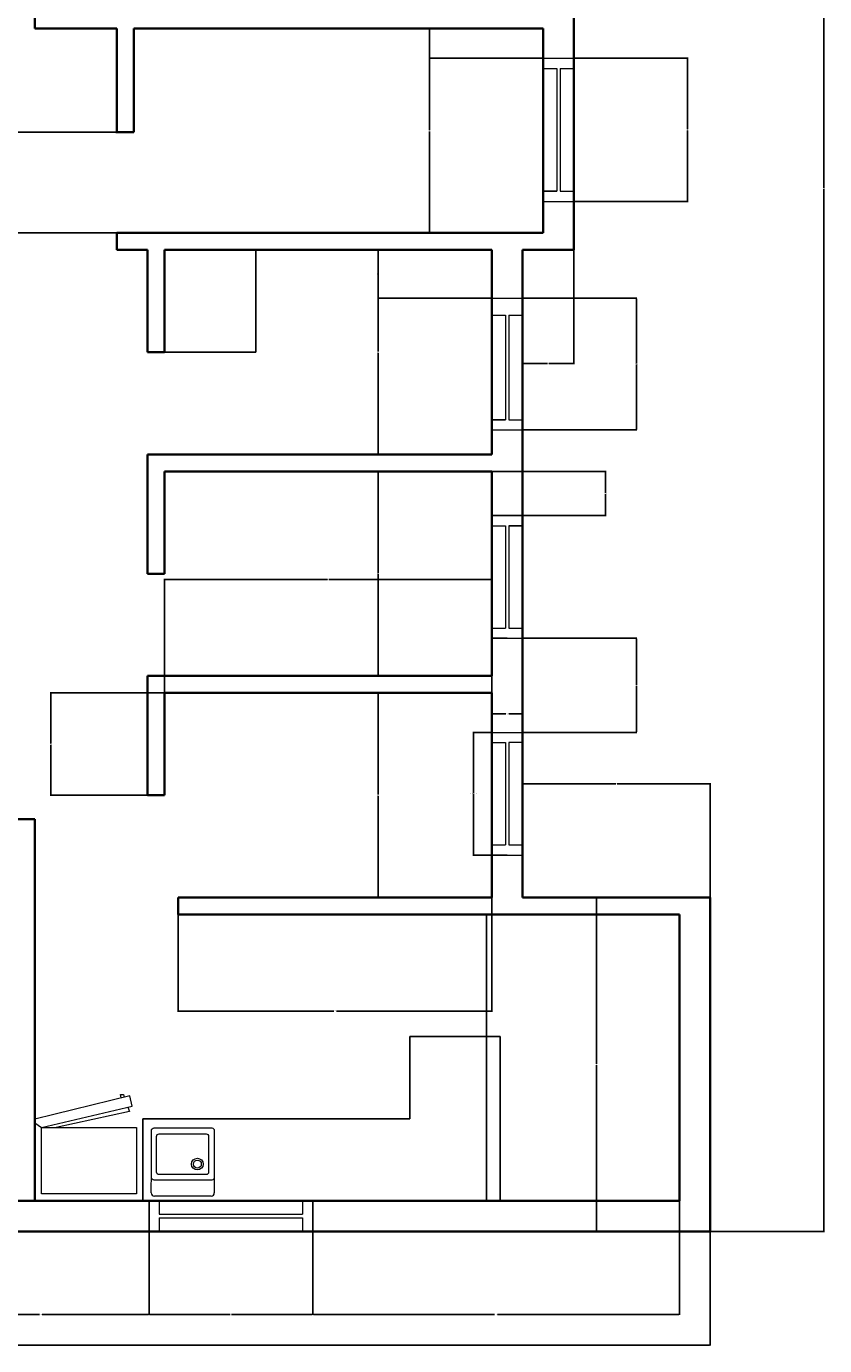
# Model space of a CAD drawing. Units: inches. Extents: x 1201 to 1750, y 1179 to 1858.
# Tile 2 of 3: x 1515 to 1750, y 1179 to 1566. Entities that reach past the tile are written whole.
import ezdxf

# ---------------------------------------------------------------- set-up
doc = ezdxf.new("R2010")
doc.units = ezdxf.units.IN
for name, color, linetype, lineweight in [('A-ANNO-DIMS', 2, 'Continuous', 18), ('A-EQPM', 8, 'Continuous', 18), ('A-FLOR-CASE', 9, 'Continuous', 25), ('A-FLOR-FIXT', 9, 'Continuous', 18), ('A-GLAZ', 4, 'Continuous', 18), ('A-WALL', 7, 'Continuous', 35)]:
    doc.layers.add(name, color=color, linetype=linetype, lineweight=lineweight)
doc.styles.get("Standard").update_dxf_attribs({"font": 'times.ttf'})
doc.dimstyles.get("Standard").update_dxf_attribs({"dimtxt": 0.18, "dimasz": 0.18, "dimexe": 0.18, "dimexo": 0.0625, "dimgap": 0.09, "dimtad": 0, "dimtih": 1, "dimtoh": 1, "dimdec": 4, "dimzin": 0, "dimdsep": 46, "dimtxsty": 'Standard', "dimcen": 0.09, "dimadec": 0, "dimazin": 0, "dimtfac": 1, "dimtdec": 4, "dimtofl": 0, "dimtmove": 0, "dimatfit": 3, "dimfxl": 1, "dimtolj": 1, "dimtzin": 0, "dimarcsym": 0})

# ---------------------------------------------------------------- blocks, each defined once
blk = doc.blocks.new('WIN-36IN')
for p, q in [((0, 36), (9, 36)), ((0, 33), (4, 33)), ((4, 33), (4, 3)), ((9, 33), (5, 33)), ((5, 33), (5, 3)), ((0, 3), (4, 3)), ((5, 3), (9, 3)), ((0, 0), (9, 0)), ((4.5, 0), (0, 0))]:
    blk.add_line(p, q)
blk = doc.blocks.new('*D5')
at = {"layer": 'A-ANNO-DIMS', "color": 0, "lineweight": -2, "transparency": 16777216}
for p, q in [((1651.92, 1358.68), (1646.41, 1358.68)), ((1646.59, 1358.5), (1646.59, 1340.86)), ((1646.59, 1322.86), (1646.59, 1340.5)), ((1651.92, 1322.68), (1646.41, 1322.68))]:
    blk.add_line(p, q, dxfattribs=at)
at = {"layer": 'A-ANNO-DIMS', "color": 0, "transparency": 16777216}
for points in [[(1646.56, 1358.5), (1646.62, 1358.5), (1646.59, 1358.68)], [(1646.56, 1322.86), (1646.62, 1322.86), (1646.59, 1322.68)]]:
    blk.add_solid(points, dxfattribs=at)
at = {"layer": 'Defpoints', "color": 0, "transparency": 16777216}
for p in [(1646.59, 1358.68), (1651.99, 1358.68), (1651.99, 1322.68)]:
    blk.add_point(p, dxfattribs=at)
at = {"layer": 'A-ANNO-DIMS', "color": 0, "transparency": 16777216, "insert": (1646.59, 1340.68), "char_height": 0.18, "attachment_point": 5}
blk.add_mtext('\\A1;WINDOW 36 TYP.', dxfattribs=at)
blk = doc.blocks.new('*D6')
at = {"layer": 'A-ANNO-DIMS', "color": 0, "lineweight": -2, "transparency": 16777216}
for p, q in [((1651.99, 1358.74), (1651.99, 1364.26)), ((1652.17, 1364.08), (1656.03, 1364.08)), ((1660.81, 1364.08), (1656.95, 1364.08)), ((1660.99, 1358.74), (1660.99, 1364.26))]:
    blk.add_line(p, q, dxfattribs=at)
at = {"layer": 'A-ANNO-DIMS', "color": 0, "transparency": 16777216}
for points in [[(1652.17, 1364.11), (1652.17, 1364.05), (1651.99, 1364.08)], [(1660.81, 1364.11), (1660.81, 1364.05), (1660.99, 1364.08)]]:
    blk.add_solid(points, dxfattribs=at)
at = {"layer": 'Defpoints', "color": 0, "transparency": 16777216}
for p in [(1660.99, 1364.08), (1651.99, 1358.68), (1660.99, 1358.68)]:
    blk.add_point(p, dxfattribs=at)
at = {"layer": 'A-ANNO-DIMS', "color": 0, "transparency": 16777216, "insert": (1656.49, 1364.08), "char_height": 0.18, "attachment_point": 5}
blk.add_mtext('\\A1;9 TYP.', dxfattribs=at)
blk = doc.blocks.new('*D7')
at = {"layer": 'A-ANNO-DIMS', "color": 0, "lineweight": -2, "transparency": 16777216}
for p, q in [((1234.99, 1212.18), (1234.99, 1178.71)), ((1715.99, 1212.18), (1715.99, 1178.71)), ((1235.17, 1178.89), (1475.22, 1178.89)), ((1715.81, 1178.89), (1475.76, 1178.89))]:
    blk.add_line(p, q, dxfattribs=at)
at = {"layer": 'A-ANNO-DIMS', "color": 0, "transparency": 16777216}
for points in [[(1235.17, 1178.92), (1235.17, 1178.86), (1234.99, 1178.89)], [(1715.81, 1178.92), (1715.81, 1178.86), (1715.99, 1178.89)]]:
    blk.add_solid(points, dxfattribs=at)
at = {"layer": 'Defpoints', "color": 0, "transparency": 16777216}
for p in [(1234.99, 1212.24), (1715.99, 1212.24), (1234.99, 1178.89)]:
    blk.add_point(p, dxfattribs=at)
at = {"layer": 'A-ANNO-DIMS', "color": 0, "transparency": 16777216, "insert": (1475.49, 1178.89), "char_height": 0.18, "attachment_point": 5}
blk.add_mtext('\\A1;481', dxfattribs=at)
blk = doc.blocks.new('*D8')
at = {"layer": 'A-ANNO-DIMS', "color": 0, "lineweight": -2, "transparency": 16777216}
for p, q in [((1676.05, 1824.24), (1749.52, 1824.24)), ((1749.34, 1824.06), (1749.34, 1518.42)), ((1749.34, 1212.42), (1749.34, 1518.06)), ((1716.05, 1212.24), (1749.52, 1212.24))]:
    blk.add_line(p, q, dxfattribs=at)
at = {"layer": 'A-ANNO-DIMS', "color": 0, "transparency": 16777216}
for points in [[(1749.31, 1824.06), (1749.37, 1824.06), (1749.34, 1824.24)], [(1749.31, 1212.42), (1749.37, 1212.42), (1749.34, 1212.24)]]:
    blk.add_solid(points, dxfattribs=at)
at = {"layer": 'Defpoints', "color": 0, "transparency": 16777216}
for p in [(1675.99, 1824.24), (1749.34, 1824.24), (1715.99, 1212.24)]:
    blk.add_point(p, dxfattribs=at)
at = {"layer": 'A-ANNO-DIMS', "color": 0, "transparency": 16777216, "insert": (1749.34, 1518.24), "char_height": 0.18, "attachment_point": 5}
blk.add_mtext('\\A1;612', dxfattribs=at)
blk = doc.blocks.new('*D14')
at = {"layer": 'A-ANNO-DIMS', "color": 0, "lineweight": -2, "transparency": 16777216}
for p, q in [((1715.92, 1310.24), (1682.46, 1310.24)), ((1682.64, 1310.06), (1682.64, 1261.42)), ((1682.64, 1212.42), (1682.64, 1261.06)), ((1715.92, 1212.24), (1682.46, 1212.24))]:
    blk.add_line(p, q, dxfattribs=at)
at = {"layer": 'A-ANNO-DIMS', "color": 0, "transparency": 16777216}
for points in [[(1682.61, 1310.06), (1682.67, 1310.06), (1682.64, 1310.24)], [(1682.61, 1212.42), (1682.67, 1212.42), (1682.64, 1212.24)]]:
    blk.add_solid(points, dxfattribs=at)
at = {"layer": 'Defpoints', "color": 0, "transparency": 16777216}
for p in [(1682.64, 1310.24), (1715.99, 1310.24), (1715.99, 1212.24)]:
    blk.add_point(p, dxfattribs=at)
at = {"layer": 'A-ANNO-DIMS', "color": 0, "transparency": 16777216, "insert": (1682.64, 1261.24), "char_height": 0.18, "attachment_point": 5}
blk.add_mtext('\\A1;98', dxfattribs=at)
blk = doc.blocks.new('*D15')
at = {"layer": 'A-ANNO-DIMS', "color": 0, "lineweight": -2, "transparency": 16777216}
for p, q in [((1660.99, 1310.3), (1660.99, 1343.77)), ((1661.17, 1343.59), (1688.28, 1343.59)), ((1715.81, 1343.59), (1688.69, 1343.59)), ((1715.99, 1310.3), (1715.99, 1343.77))]:
    blk.add_line(p, q, dxfattribs=at)
at = {"layer": 'A-ANNO-DIMS', "color": 0, "transparency": 16777216}
for points in [[(1661.17, 1343.62), (1661.17, 1343.56), (1660.99, 1343.59)], [(1715.81, 1343.62), (1715.81, 1343.56), (1715.99, 1343.59)]]:
    blk.add_solid(points, dxfattribs=at)
at = {"layer": 'Defpoints', "color": 0, "transparency": 16777216}
for p in [(1715.99, 1343.59), (1660.99, 1310.24), (1715.99, 1310.24)]:
    blk.add_point(p, dxfattribs=at)
at = {"layer": 'A-ANNO-DIMS', "color": 0, "transparency": 16777216, "insert": (1688.49, 1343.59), "char_height": 0.18, "attachment_point": 5}
blk.add_mtext('\\A1;55', dxfattribs=at)
blk = doc.blocks.new('*D16')
at = {"layer": 'A-ANNO-DIMS', "color": 0, "lineweight": -2, "transparency": 16777216}
for p, q in [((1660.99, 1500.18), (1660.99, 1466.71)), ((1675.99, 1500.18), (1675.99, 1466.71)), ((1661.17, 1466.89), (1668.29, 1466.89)), ((1675.81, 1466.89), (1668.69, 1466.89))]:
    blk.add_line(p, q, dxfattribs=at)
at = {"layer": 'A-ANNO-DIMS', "color": 0, "transparency": 16777216}
for points in [[(1661.17, 1466.92), (1661.17, 1466.86), (1660.99, 1466.89)], [(1675.81, 1466.92), (1675.81, 1466.86), (1675.99, 1466.89)]]:
    blk.add_solid(points, dxfattribs=at)
at = {"layer": 'Defpoints', "color": 0, "transparency": 16777216}
for p in [(1660.99, 1500.24), (1675.99, 1500.24), (1660.99, 1466.89)]:
    blk.add_point(p, dxfattribs=at)
at = {"layer": 'A-ANNO-DIMS', "color": 0, "transparency": 16777216, "insert": (1668.49, 1466.89), "char_height": 0.18, "attachment_point": 5}
blk.add_mtext('\\A1;15', dxfattribs=at)
blk = doc.blocks.new('*D17')
at = {"layer": 'A-ANNO-DIMS', "color": 0, "lineweight": -2, "transparency": 16777216}
for p, q in [((1666.92, 1565.24), (1633.46, 1565.24)), ((1633.64, 1565.06), (1633.64, 1535.42)), ((1633.64, 1505.42), (1633.64, 1535.06)), ((1666.92, 1505.24), (1633.46, 1505.24))]:
    blk.add_line(p, q, dxfattribs=at)
at = {"layer": 'A-ANNO-DIMS', "color": 0, "transparency": 16777216}
for points in [[(1633.61, 1565.06), (1633.67, 1565.06), (1633.64, 1565.24)], [(1633.61, 1505.42), (1633.67, 1505.42), (1633.64, 1505.24)]]:
    blk.add_solid(points, dxfattribs=at)
at = {"layer": 'Defpoints', "color": 0, "transparency": 16777216}
for p in [(1633.64, 1565.24), (1666.99, 1565.24), (1666.99, 1505.24)]:
    blk.add_point(p, dxfattribs=at)
at = {"layer": 'A-ANNO-DIMS', "color": 0, "transparency": 16777216, "insert": (1633.64, 1535.24), "char_height": 0.18, "attachment_point": 5}
blk.add_mtext('\\A1;60', dxfattribs=at)
blk = doc.blocks.new('*D20')
at = {"layer": 'A-ANNO-DIMS', "color": 0, "lineweight": -2, "transparency": 16777216}
for p, q in [((1555.99, 1370.3), (1555.99, 1403.77)), ((1556.17, 1403.59), (1603.77, 1403.59)), ((1651.81, 1403.59), (1604.2, 1403.59)), ((1651.99, 1370.3), (1651.99, 1403.77))]:
    blk.add_line(p, q, dxfattribs=at)
at = {"layer": 'A-ANNO-DIMS', "color": 0, "transparency": 16777216}
for points in [[(1556.17, 1403.62), (1556.17, 1403.56), (1555.99, 1403.59)], [(1651.81, 1403.62), (1651.81, 1403.56), (1651.99, 1403.59)]]:
    blk.add_solid(points, dxfattribs=at)
at = {"layer": 'Defpoints', "color": 0, "transparency": 16777216}
for p in [(1651.99, 1403.59), (1555.99, 1370.24), (1651.99, 1370.24)]:
    blk.add_point(p, dxfattribs=at)
at = {"layer": 'A-ANNO-DIMS', "color": 0, "transparency": 16777216, "insert": (1603.99, 1403.59), "char_height": 0.18, "attachment_point": 5}
blk.add_mtext('\\A1;96', dxfattribs=at)
blk = doc.blocks.new('*D21')
at = {"layer": 'A-ANNO-DIMS', "color": 0, "lineweight": -2, "transparency": 16777216}
for p, q in [((1651.92, 1370.24), (1618.46, 1370.24)), ((1618.64, 1370.06), (1618.64, 1340.42)), ((1618.64, 1310.42), (1618.64, 1340.06)), ((1651.92, 1310.24), (1618.46, 1310.24))]:
    blk.add_line(p, q, dxfattribs=at)
at = {"layer": 'A-ANNO-DIMS', "color": 0, "transparency": 16777216}
for points in [[(1618.61, 1370.06), (1618.67, 1370.06), (1618.64, 1370.24)], [(1618.61, 1310.42), (1618.67, 1310.42), (1618.64, 1310.24)]]:
    blk.add_solid(points, dxfattribs=at)
at = {"layer": 'Defpoints', "color": 0, "transparency": 16777216}
for p in [(1618.64, 1370.24), (1651.99, 1370.24), (1651.99, 1310.24)]:
    blk.add_point(p, dxfattribs=at)
at = {"layer": 'A-ANNO-DIMS', "color": 0, "transparency": 16777216, "insert": (1618.64, 1340.24), "char_height": 0.18, "attachment_point": 5}
blk.add_mtext('\\A1;60', dxfattribs=at)
blk = doc.blocks.new('*D22')
at = {"layer": 'A-ANNO-DIMS', "color": 0, "lineweight": -2, "transparency": 16777216}
for p, q in [((1651.92, 1435.24), (1618.46, 1435.24)), ((1618.64, 1435.06), (1618.64, 1405.42)), ((1618.64, 1375.42), (1618.64, 1405.06)), ((1651.92, 1375.24), (1618.46, 1375.24))]:
    blk.add_line(p, q, dxfattribs=at)
at = {"layer": 'A-ANNO-DIMS', "color": 0, "transparency": 16777216}
for points in [[(1618.61, 1435.06), (1618.67, 1435.06), (1618.64, 1435.24)], [(1618.61, 1375.42), (1618.67, 1375.42), (1618.64, 1375.24)]]:
    blk.add_solid(points, dxfattribs=at)
at = {"layer": 'Defpoints', "color": 0, "transparency": 16777216}
for p in [(1618.64, 1435.24), (1651.99, 1435.24), (1651.99, 1375.24)]:
    blk.add_point(p, dxfattribs=at)
at = {"layer": 'A-ANNO-DIMS', "color": 0, "transparency": 16777216, "insert": (1618.64, 1405.24), "char_height": 0.18, "attachment_point": 5}
blk.add_mtext('\\A1;60', dxfattribs=at)
blk = doc.blocks.new('*D23')
at = {"layer": 'A-ANNO-DIMS', "color": 0, "lineweight": -2, "transparency": 16777216}
for p, q in [((1651.92, 1500.24), (1618.46, 1500.24)), ((1618.64, 1500.06), (1618.64, 1470.42)), ((1618.64, 1440.42), (1618.64, 1470.06)), ((1651.92, 1440.24), (1618.46, 1440.24))]:
    blk.add_line(p, q, dxfattribs=at)
at = {"layer": 'A-ANNO-DIMS', "color": 0, "transparency": 16777216}
for points in [[(1618.61, 1500.06), (1618.67, 1500.06), (1618.64, 1500.24)], [(1618.61, 1440.42), (1618.67, 1440.42), (1618.64, 1440.24)]]:
    blk.add_solid(points, dxfattribs=at)
at = {"layer": 'Defpoints', "color": 0, "transparency": 16777216}
for p in [(1618.64, 1500.24), (1651.99, 1500.24), (1651.99, 1440.24)]:
    blk.add_point(p, dxfattribs=at)
at = {"layer": 'A-ANNO-DIMS', "color": 0, "transparency": 16777216, "insert": (1618.64, 1470.24), "char_height": 0.18, "attachment_point": 5}
blk.add_mtext('\\A1;60', dxfattribs=at)
blk = doc.blocks.new('*D33')
at = {"layer": 'A-ANNO-DIMS', "color": 0, "lineweight": -2, "transparency": 16777216}
for p, q in [((1476.42, 1565.3), (1476.42, 1598.77)), ((1476.6, 1598.59), (1496.82, 1598.59)), ((1517.81, 1598.59), (1497.58, 1598.59)), ((1517.99, 1565.3), (1517.99, 1598.77))]:
    blk.add_line(p, q, dxfattribs=at)
at = {"layer": 'A-ANNO-DIMS', "color": 0, "transparency": 16777216}
for points in [[(1476.6, 1598.62), (1476.6, 1598.56), (1476.42, 1598.59)], [(1517.81, 1598.62), (1517.81, 1598.56), (1517.99, 1598.59)]]:
    blk.add_solid(points, dxfattribs=at)
at = {"layer": 'Defpoints', "color": 0, "transparency": 16777216}
for p in [(1517.99, 1598.59), (1476.42, 1565.24), (1517.99, 1565.24)]:
    blk.add_point(p, dxfattribs=at)
at = {"layer": 'A-ANNO-DIMS', "color": 0, "transparency": 16777216, "insert": (1497.2, 1598.59), "char_height": 0.18, "attachment_point": 5}
blk.add_mtext('\\A1;41.57', dxfattribs=at)
blk = doc.blocks.new('*D42')
at = {"layer": 'A-ANNO-DIMS', "color": 0, "lineweight": -2, "transparency": 16777216}
for p, q in [((1487.97, 1221.18), (1487.97, 1187.71)), ((1551.45, 1221.18), (1551.45, 1187.71)), ((1488.15, 1187.89), (1519.33, 1187.89)), ((1551.27, 1187.89), (1520.09, 1187.89))]:
    blk.add_line(p, q, dxfattribs=at)
at = {"layer": 'A-ANNO-DIMS', "color": 0, "transparency": 16777216}
for points in [[(1488.15, 1187.92), (1488.15, 1187.86), (1487.97, 1187.89)], [(1551.27, 1187.92), (1551.27, 1187.86), (1551.45, 1187.89)]]:
    blk.add_solid(points, dxfattribs=at)
at = {"layer": 'Defpoints', "color": 0, "transparency": 16777216}
for p in [(1487.97, 1221.24), (1551.45, 1221.24), (1487.97, 1187.89)]:
    blk.add_point(p, dxfattribs=at)
at = {"layer": 'A-ANNO-DIMS', "color": 0, "transparency": 16777216, "insert": (1519.71, 1187.89), "char_height": 0.18, "attachment_point": 5}
blk.add_mtext('\\A1;63.48', dxfattribs=at)
blk = doc.blocks.new('*D43')
at = {"layer": 'A-ANNO-DIMS', "color": 0, "lineweight": -2, "transparency": 16777216}
for p, q in [((1551.45, 1221.18), (1551.45, 1187.71)), ((1599.45, 1221.18), (1599.45, 1187.71)), ((1551.63, 1187.89), (1575.23, 1187.89)), ((1599.27, 1187.89), (1575.66, 1187.89))]:
    blk.add_line(p, q, dxfattribs=at)
at = {"layer": 'A-ANNO-DIMS', "color": 0, "transparency": 16777216}
for points in [[(1551.63, 1187.92), (1551.63, 1187.86), (1551.45, 1187.89)], [(1599.27, 1187.92), (1599.27, 1187.86), (1599.45, 1187.89)]]:
    blk.add_solid(points, dxfattribs=at)
at = {"layer": 'Defpoints', "color": 0, "transparency": 16777216}
for p in [(1551.45, 1221.24), (1599.45, 1221.24), (1551.45, 1187.89)]:
    blk.add_point(p, dxfattribs=at)
at = {"layer": 'A-ANNO-DIMS', "color": 0, "transparency": 16777216, "insert": (1575.45, 1187.89), "char_height": 0.18, "attachment_point": 5}
blk.add_mtext('\\A1;48', dxfattribs=at)
blk = doc.blocks.new('*D44')
at = {"layer": 'A-ANNO-DIMS', "color": 0, "lineweight": -2, "transparency": 16777216}
for p, q in [((1599.45, 1221.18), (1599.45, 1187.71)), ((1706.99, 1221.18), (1706.99, 1187.71)), ((1599.63, 1187.89), (1652.78, 1187.89)), ((1706.81, 1187.89), (1653.65, 1187.89))]:
    blk.add_line(p, q, dxfattribs=at)
at = {"layer": 'A-ANNO-DIMS', "color": 0, "transparency": 16777216}
for points in [[(1599.63, 1187.92), (1599.63, 1187.86), (1599.45, 1187.89)], [(1706.81, 1187.92), (1706.81, 1187.86), (1706.99, 1187.89)]]:
    blk.add_solid(points, dxfattribs=at)
at = {"layer": 'Defpoints', "color": 0, "transparency": 16777216}
for p in [(1599.45, 1221.24), (1706.99, 1221.24), (1599.45, 1187.89)]:
    blk.add_point(p, dxfattribs=at)
at = {"layer": 'A-ANNO-DIMS', "color": 0, "transparency": 16777216, "insert": (1653.22, 1187.89), "char_height": 0.18, "attachment_point": 5}
blk.add_mtext('\\A1;107.54', dxfattribs=at)
blk = doc.blocks.new('*D50')
at = {"layer": 'A-ANNO-DIMS', "color": 0, "lineweight": -2, "transparency": 16777216}
for p, q in [((1541.92, 1534.83), (1508.46, 1534.83)), ((1508.64, 1534.65), (1508.64, 1520.22)), ((1508.64, 1505.42), (1508.64, 1519.85)), ((1541.92, 1505.24), (1508.46, 1505.24))]:
    blk.add_line(p, q, dxfattribs=at)
at = {"layer": 'A-ANNO-DIMS', "color": 0, "transparency": 16777216}
for points in [[(1508.61, 1534.65), (1508.67, 1534.65), (1508.64, 1534.83)], [(1508.61, 1505.42), (1508.67, 1505.42), (1508.64, 1505.24)]]:
    blk.add_solid(points, dxfattribs=at)
at = {"layer": 'Defpoints', "color": 0, "transparency": 16777216}
for p in [(1508.64, 1534.83), (1541.99, 1534.83), (1541.99, 1505.24)]:
    blk.add_point(p, dxfattribs=at)
at = {"layer": 'A-ANNO-DIMS', "color": 0, "transparency": 16777216, "insert": (1508.64, 1520.03), "char_height": 0.18, "attachment_point": 5}
blk.add_mtext('\\A1;29.585', dxfattribs=at)
blk = doc.blocks.new('*D51')
at = {"layer": 'A-ANNO-DIMS', "color": 0, "lineweight": -2, "transparency": 16777216}
for p, q in [((1555.92, 1370.24), (1522.46, 1370.24)), ((1522.64, 1370.06), (1522.64, 1355.42)), ((1522.64, 1340.42), (1522.64, 1355.06)), ((1555.92, 1340.24), (1522.46, 1340.24))]:
    blk.add_line(p, q, dxfattribs=at)
at = {"layer": 'A-ANNO-DIMS', "color": 0, "transparency": 16777216}
for points in [[(1522.61, 1370.06), (1522.67, 1370.06), (1522.64, 1370.24)], [(1522.61, 1340.42), (1522.67, 1340.42), (1522.64, 1340.24)]]:
    blk.add_solid(points, dxfattribs=at)
at = {"layer": 'Defpoints', "color": 0, "transparency": 16777216}
for p in [(1522.64, 1370.24), (1555.99, 1370.24), (1555.99, 1340.24)]:
    blk.add_point(p, dxfattribs=at)
at = {"layer": 'A-ANNO-DIMS', "color": 0, "transparency": 16777216, "insert": (1522.64, 1355.24), "char_height": 0.18, "attachment_point": 5}
blk.add_mtext('\\A1;30', dxfattribs=at)
blk = doc.blocks.new('*D52')
at = {"layer": 'A-ANNO-DIMS', "color": 0, "lineweight": -2, "transparency": 16777216}
for p, q in [((1661.05, 1386.31), (1694.52, 1386.31)), ((1694.34, 1386.13), (1694.34, 1372.67)), ((1694.34, 1358.86), (1694.34, 1372.31)), ((1661.05, 1358.68), (1694.52, 1358.68))]:
    blk.add_line(p, q, dxfattribs=at)
at = {"layer": 'A-ANNO-DIMS', "color": 0, "transparency": 16777216}
for points in [[(1694.31, 1386.13), (1694.37, 1386.13), (1694.34, 1386.31)], [(1694.31, 1358.86), (1694.37, 1358.86), (1694.34, 1358.68)]]:
    blk.add_solid(points, dxfattribs=at)
at = {"layer": 'Defpoints', "color": 0, "transparency": 16777216}
for p in [(1660.99, 1386.31), (1660.99, 1358.68), (1694.34, 1358.68)]:
    blk.add_point(p, dxfattribs=at)
at = {"layer": 'A-ANNO-DIMS', "color": 0, "transparency": 16777216, "insert": (1694.34, 1372.49), "char_height": 0.18, "attachment_point": 5}
blk.add_mtext('\\A1;27.63', dxfattribs=at)
blk = doc.blocks.new('*D53')
at = {"layer": 'A-ANNO-DIMS', "color": 0, "lineweight": -2, "transparency": 16777216}
for p, q in [((1652.05, 1435.24), (1685.52, 1435.24)), ((1685.34, 1435.06), (1685.34, 1428.96)), ((1685.34, 1422.49), (1685.34, 1428.59)), ((1652.05, 1422.31), (1685.52, 1422.31))]:
    blk.add_line(p, q, dxfattribs=at)
at = {"layer": 'A-ANNO-DIMS', "color": 0, "transparency": 16777216}
for points in [[(1685.31, 1435.06), (1685.37, 1435.06), (1685.34, 1435.24)], [(1685.31, 1422.49), (1685.37, 1422.49), (1685.34, 1422.31)]]:
    blk.add_solid(points, dxfattribs=at)
at = {"layer": 'Defpoints', "color": 0, "transparency": 16777216}
for p in [(1651.99, 1435.24), (1651.99, 1422.31), (1685.34, 1422.31)]:
    blk.add_point(p, dxfattribs=at)
at = {"layer": 'A-ANNO-DIMS', "color": 0, "transparency": 16777216, "insert": (1685.34, 1428.77), "char_height": 0.18, "attachment_point": 5}
blk.add_mtext('\\A1;12.936', dxfattribs=at)
blk = doc.blocks.new('*D54')
at = {"layer": 'A-ANNO-DIMS', "color": 0, "lineweight": -2, "transparency": 16777216}
for p, q in [((1661.05, 1486.12), (1694.52, 1486.12)), ((1694.34, 1485.94), (1694.34, 1466.95)), ((1694.34, 1447.6), (1694.34, 1466.59)), ((1661.05, 1447.42), (1694.52, 1447.42))]:
    blk.add_line(p, q, dxfattribs=at)
at = {"layer": 'A-ANNO-DIMS', "color": 0, "transparency": 16777216}
for points in [[(1694.31, 1485.94), (1694.37, 1485.94), (1694.34, 1486.12)], [(1694.31, 1447.6), (1694.37, 1447.6), (1694.34, 1447.42)]]:
    blk.add_solid(points, dxfattribs=at)
at = {"layer": 'Defpoints', "color": 0, "transparency": 16777216}
for p in [(1660.99, 1486.12), (1660.99, 1447.42), (1694.34, 1447.42)]:
    blk.add_point(p, dxfattribs=at)
at = {"layer": 'A-ANNO-DIMS', "color": 0, "transparency": 16777216, "insert": (1694.34, 1466.77), "char_height": 0.18, "attachment_point": 5}
blk.add_mtext('\\A1;38.695', dxfattribs=at)
blk = doc.blocks.new('*D55')
at = {"layer": 'A-ANNO-DIMS', "color": 0, "lineweight": -2, "transparency": 16777216}
for p, q in [((1651.92, 1500.24), (1618.46, 1500.24)), ((1618.64, 1500.06), (1618.64, 1493.36)), ((1618.64, 1486.3), (1618.64, 1493)), ((1651.92, 1486.12), (1618.46, 1486.12))]:
    blk.add_line(p, q, dxfattribs=at)
at = {"layer": 'A-ANNO-DIMS', "color": 0, "transparency": 16777216}
for points in [[(1618.61, 1500.06), (1618.67, 1500.06), (1618.64, 1500.24)], [(1618.61, 1486.3), (1618.67, 1486.3), (1618.64, 1486.12)]]:
    blk.add_solid(points, dxfattribs=at)
at = {"layer": 'Defpoints', "color": 0, "transparency": 16777216}
for p in [(1618.64, 1500.24), (1651.99, 1500.24), (1651.99, 1486.12)]:
    blk.add_point(p, dxfattribs=at)
at = {"layer": 'A-ANNO-DIMS', "color": 0, "transparency": 16777216, "insert": (1618.64, 1493.18), "char_height": 0.18, "attachment_point": 5}
blk.add_mtext('\\A1;14.122', dxfattribs=at)
blk = doc.blocks.new('*D56')
at = {"layer": 'A-ANNO-DIMS', "color": 0, "lineweight": -2, "transparency": 16777216}
for p, q in [((1666.92, 1565.24), (1633.46, 1565.24)), ((1633.64, 1565.06), (1633.64, 1561.05)), ((1633.64, 1556.67), (1633.64, 1560.68)), ((1666.92, 1556.49), (1633.46, 1556.49))]:
    blk.add_line(p, q, dxfattribs=at)
at = {"layer": 'A-ANNO-DIMS', "color": 0, "transparency": 16777216}
for points in [[(1633.61, 1565.06), (1633.67, 1565.06), (1633.64, 1565.24)], [(1633.61, 1556.67), (1633.67, 1556.67), (1633.64, 1556.49)]]:
    blk.add_solid(points, dxfattribs=at)
at = {"layer": 'Defpoints', "color": 0, "transparency": 16777216}
for p in [(1633.64, 1565.24), (1666.99, 1565.24), (1666.99, 1556.49)]:
    blk.add_point(p, dxfattribs=at)
at = {"layer": 'A-ANNO-DIMS', "color": 0, "transparency": 16777216, "insert": (1633.64, 1560.87), "char_height": 0.18, "attachment_point": 5}
blk.add_mtext('\\A1;8.751', dxfattribs=at)
blk = doc.blocks.new('*D57')
at = {"layer": 'A-ANNO-DIMS', "color": 0, "lineweight": -2, "transparency": 16777216}
for p, q in [((1676.049469, 1556.490677), (1709.516969, 1556.490677)), ((1709.336969, 1556.310677), (1709.336969, 1535.670677)), ((1709.336969, 1514.670677), (1709.336969, 1535.310677)), ((1676.049469, 1514.490677), (1709.516969, 1514.490677))]:
    blk.add_line(p, q, dxfattribs=at)
at = {"layer": 'A-ANNO-DIMS', "color": 0, "transparency": 16777216}
for points in [[(1709.306969, 1556.310677), (1709.366969, 1556.310677), (1709.336969, 1556.490677)], [(1709.306969, 1514.670677), (1709.366969, 1514.670677), (1709.336969, 1514.490677)]]:
    blk.add_solid(points, dxfattribs=at)
at = {"layer": 'Defpoints', "color": 0, "transparency": 16777216}
for p in [(1675.986969, 1556.490677), (1675.986969, 1514.490677), (1709.336969, 1514.490677)]:
    blk.add_point(p, dxfattribs=at)
at = {"layer": 'A-ANNO-DIMS', "color": 0, "transparency": 16777216, "insert": (1709.336969, 1535.490677), "char_height": 0.18, "attachment_point": 5}
blk.add_mtext('\\A1;42', dxfattribs=at)
blk = doc.blocks.new('*D60')
at = {"layer": 'A-ANNO-DIMS', "color": 0, "lineweight": -2, "transparency": 16777216}
for p, q in [((1560, 1310.18), (1560, 1276.71)), ((1651.99, 1310.18), (1651.99, 1276.71)), ((1560.18, 1276.89), (1605.62, 1276.89)), ((1651.81, 1276.89), (1606.37, 1276.89))]:
    blk.add_line(p, q, dxfattribs=at)
at = {"layer": 'A-ANNO-DIMS', "color": 0, "transparency": 16777216}
for points in [[(1560.18, 1276.92), (1560.18, 1276.86), (1560, 1276.89)], [(1651.81, 1276.92), (1651.81, 1276.86), (1651.99, 1276.89)]]:
    blk.add_solid(points, dxfattribs=at)
at = {"layer": 'Defpoints', "color": 0, "transparency": 16777216}
for p in [(1560, 1310.24), (1651.99, 1310.24), (1560, 1276.89)]:
    blk.add_point(p, dxfattribs=at)
at = {"layer": 'A-ANNO-DIMS', "color": 0, "transparency": 16777216, "insert": (1606, 1276.89), "char_height": 0.18, "attachment_point": 5}
blk.add_mtext('\\A1;91.98', dxfattribs=at)

msp = doc.modelspace()

# ---------------------------------------------------------------- linework, layer by layer
at = {"layer": 'A-EQPM'}
for p, q in [((1545.83, 1252.0277), (1517.987, 1245.1657)), ((1543.2936, 1251.4026), (1543.0407, 1252.4137)), ((1543.0407, 1252.4137), (1543.922, 1252.4137)), ((1543.922, 1252.4137), (1544.1209, 1251.6065)), ((1546.5419, 1248.9648), (1545.83, 1252.0277)), ((1519.8818, 1242.7682), (1546.5419, 1248.9648)), ((1545.6986, 1247.4657), (1524.2446, 1242.7682)), ((1545.244, 1248.6631), (1545.6986, 1247.4657)), ((1517.987, 1244.1019), (1519.8818, 1242.7682))]:
    msp.add_line(p, q, dxfattribs=at)
msp.add_lwpolyline([(1519.8818, 1242.7682), (1547.7559, 1242.7682), (1547.7559, 1223.2693), (1519.8818, 1223.2693)], close=True, dxfattribs=at)
at = {"layer": 'A-FLOR-CASE'}
for p, q in [((1582.7178, 1500.2419), (1582.7178, 1470.2419)), ((1582.7178, 1470.2419), (1555.987, 1470.2419)), ((1650.3922, 1305.2419), (1650.3922, 1221.2419)), ((1654.3922, 1269.4716), (1627.8765, 1269.4716)), ((1627.8765, 1269.4716), (1627.8765, 1245.2419)), ((1641.6906, 1269.4716), (1654.3922, 1269.4716)), ((1654.3922, 1269.4716), (1654.3922, 1221.2419)), ((1549.6518, 1245.2419), (1627.8765, 1245.2419)), ((1549.6518, 1245.2419), (1549.6518, 1221.2419))]:
    msp.add_line(p, q, dxfattribs=at)
at = {"layer": 'A-FLOR-FIXT'}
for p, q in [((1552.1166, 1223.5146), (1552.1422, 1229.7768)), ((1570.5924, 1230.55), (1570.5924, 1223.5146)), ((1569.6604, 1222.5826), (1553.0485, 1222.5826))]:
    msp.add_line(p, q, dxfattribs=at)
for points in [[(1552.9079, 1242.6008), (1569.8267, 1242.6008, -0.41421356), (1570.5924, 1241.835), (1570.5924, 1228.0744, -0.41421356), (1569.8267, 1227.3086), (1552.9079, 1227.3086, -0.41421356), (1552.1422, 1228.0744), (1552.1422, 1241.835, -0.41421356)], [(1554.3944, 1240.8531), (1568.1653, 1240.8531, -0.41421356), (1568.931, 1240.0873), (1568.931, 1229.6473, -0.41421356), (1568.1653, 1228.8815), (1554.3944, 1228.8815, -0.41421356), (1553.6287, 1229.6473), (1553.6287, 1240.0873, -0.41421356)]]:
    msp.add_lwpolyline(points, format="xyb", close=True, dxfattribs=at)
for radius in [1.7171, 1.1648]:
    msp.add_circle((1565.6113, 1231.9714), radius, dxfattribs=at)
for centre, start, end in [((1553.0485, 1223.5146), 180, 270), ((1569.6604, 1223.5146), 270, 0)]:
    msp.add_arc(centre, 0.932, start, end, dxfattribs=at)
at = {"layer": 'A-GLAZ'}
for p, q in [((1666.987, 1556.4907), (1675.987, 1556.4907)), ((1666.987, 1553.4907), (1670.987, 1553.4907)), ((1670.987, 1553.4907), (1670.987, 1517.4907)), ((1671.987, 1553.4907), (1671.987, 1517.4907)), ((1671.987, 1553.4907), (1675.987, 1553.4907)), ((1670.987, 1517.4907), (1666.987, 1517.4907)), ((1666.987, 1517.4907), (1670.987, 1517.4907)), ((1666.987, 1514.4907), (1675.987, 1514.4907)), ((1671.987, 1517.4907), (1675.987, 1517.4907)), ((1651.987, 1486.1199), (1660.987, 1486.1199)), ((1651.987, 1481.1199), (1655.987, 1481.1199)), ((1655.987, 1481.1199), (1655.987, 1450.425)), ((1656.987, 1481.1199), (1656.987, 1450.425)), ((1656.987, 1481.1199), (1660.987, 1481.1199)), ((1655.987, 1450.425), (1651.987, 1450.425)), ((1651.987, 1450.425), (1655.987, 1450.425)), ((1656.987, 1450.425), (1660.987, 1450.425)), ((1651.987, 1447.425), (1660.987, 1447.425)), ((1660.987, 1422.3054), (1656.487, 1422.3054)), ((1656.987, 1419.3054), (1660.987, 1419.3054)), ((1551.4478, 1221.2419), (1551.4478, 1212.2419)), ((1554.4478, 1221.2419), (1554.4478, 1217.2419)), ((1596.4478, 1221.2419), (1596.4478, 1217.2419)), ((1599.4478, 1216.7419), (1599.4478, 1221.2419)), ((1599.4478, 1221.2419), (1599.4478, 1212.2419)), ((1554.4478, 1217.2419), (1596.4478, 1217.2419)), ((1554.4478, 1216.2419), (1596.4478, 1216.2419)), ((1554.4478, 1216.2419), (1554.4478, 1212.2419)), ((1596.4478, 1216.2419), (1596.4478, 1212.2419))]:
    msp.add_line(p, q, dxfattribs=at)
at = {"layer": 'A-WALL'}
for p, q in [((1517.987, 1612.2419), (1517.987, 1565.2419)), ((1517.987, 1570.2419), (1517.987, 1565.2419)), ((1517.987, 1570.2419), (1517.987, 1565.2419)), ((1675.987, 1571.1497), (1675.987, 1500.2419)), ((1517.987, 1565.2419), (1541.987, 1565.2419)), ((1541.987, 1565.2419), (1541.987, 1534.5024)), ((1541.987, 1565.2419), (1541.987, 1534.8271)), ((1546.987, 1565.2419), (1546.987, 1534.8271)), ((1546.987, 1565.2419), (1546.987, 1534.8271)), ((1546.987, 1565.2419), (1666.987, 1565.2419)), ((1666.987, 1565.2419), (1666.987, 1505.2419)), ((1541.987, 1534.8271), (1546.987, 1534.8271)), ((1541.987, 1505.2419), (1666.987, 1505.2419)), ((1541.987, 1505.2419), (1541.987, 1500.2419)), ((1541.987, 1500.2419), (1550.987, 1500.2419)), ((1550.987, 1500.2419), (1550.987, 1470.2419)), ((1555.987, 1500.2419), (1555.987, 1470.2419)), ((1555.987, 1500.2419), (1651.987, 1500.2419)), ((1651.987, 1500.2419), (1651.987, 1440.2419)), ((1675.987, 1500.2419), (1660.987, 1500.2419)), ((1660.987, 1500.2419), (1660.987, 1310.2419)), ((1660.987, 1500.2419), (1675.987, 1500.2419)), ((1553.8963, 1470.2419), (1550.987, 1470.2419)), ((1550.987, 1470.2419), (1555.987, 1470.2419)), ((1651.987, 1440.2419), (1550.987, 1440.2419)), ((1550.987, 1440.2419), (1550.987, 1405.2419)), ((1651.987, 1435.2419), (1555.987, 1435.2419)), ((1555.987, 1435.2419), (1555.987, 1405.2419)), ((1651.987, 1435.2419), (1651.987, 1375.2419)), ((1553.1857, 1405.2419), (1550.987, 1405.2419)), ((1550.987, 1405.2419), (1555.987, 1405.2419)), ((1651.987, 1375.2419), (1550.987, 1375.2419)), ((1550.987, 1375.2419), (1550.987, 1340.2419)), ((1651.987, 1370.2419), (1555.987, 1370.2419)), ((1555.987, 1370.2419), (1555.987, 1340.2419)), ((1651.987, 1370.2419), (1651.987, 1310.2419)), ((1553.28, 1340.2419), (1550.987, 1340.2419)), ((1550.987, 1340.2419), (1555.987, 1340.2419)), ((1434.987, 1333.2419), (1517.987, 1333.2419)), ((1517.987, 1305.2419), (1517.987, 1333.2419)), ((1651.987, 1310.2419), (1560.0046, 1310.2419)), ((1560.0046, 1307.8991), (1560.0046, 1310.2419)), ((1560.0046, 1310.2419), (1560.0046, 1305.2419)), ((1715.987, 1310.2419), (1660.987, 1310.2419)), ((1715.987, 1310.2419), (1715.987, 1212.2419)), ((1517.987, 1305.2419), (1517.987, 1221.2419)), ((1706.987, 1305.2419), (1560.0046, 1305.2419)), ((1706.987, 1305.2419), (1706.987, 1221.2419)), ((1706.987, 1221.2419), (1243.987, 1221.2419)), ((1517.987, 1221.2419), (1706.987, 1221.2419)), ((1715.987, 1212.2419), (1234.987, 1212.2419))]:
    msp.add_line(p, q, dxfattribs=at)

# ---------------------------------------------------------------- block references
at = {"layer": 'A-GLAZ'}
for p in [(1651.987, 1386.3054), (1651.987, 1322.6779)]:
    msp.add_blockref('WIN-36IN', p, dxfattribs=at)

# ---------------------------------------------------------------- dimensions: what is measured, and where the dimension line sits
at = {"layer": 'A-ANNO-DIMS'}
for base, p1, p2, angle, override, picture, middle in [((1749.337, 1824.2419), (1715.987, 1212.2419), (1675.987, 1824.2419), 90, {"dimdec": 0, "dimlfac": 1, "dimrnd": 0, "dimzin": 0, "dimdsep": 46, "dimlunit": 2}, '*D8', (1749.337, 1518.2419)), ((1633.637, 1565.2419), (1666.987, 1556.4907), (1666.987, 1565.2419), 90, {"dimdec": 3, "dimlfac": 1, "dimrnd": 0, "dimzin": 0, "dimdsep": 46, "dimlunit": 2}, '*D56', (1633.637, 1560.8663)), ((1633.637, 1565.2419), (1666.987, 1505.2419), (1666.987, 1565.2419), 90, {"dimdec": 0, "dimlfac": 1, "dimrnd": 0, "dimzin": 0, "dimdsep": 46, "dimlunit": 2}, '*D17', (1633.637, 1535.2419)), ((1709.337, 1514.4907), (1675.987, 1556.4907), (1675.987, 1514.4907), 270, {"dimdec": 0, "dimlfac": 1, "dimrnd": 0, "dimzin": 0, "dimdsep": 46, "dimlunit": 2}, '*D57', (1709.337, 1535.4907)), ((1508.637, 1534.8271), (1541.987, 1505.2419), (1541.987, 1534.8271), 90, {"dimdec": 3, "dimlfac": 1, "dimrnd": 0, "dimzin": 0, "dimdsep": 46, "dimlunit": 2}, '*D50', (1508.637, 1520.0345)), ((1618.637, 1500.2419), (1651.987, 1486.1199), (1651.987, 1500.2419), 90, {"dimdec": 3, "dimlfac": 1, "dimrnd": 0, "dimzin": 0, "dimdsep": 46, "dimlunit": 2}, '*D55', (1618.637, 1493.1809)), ((1618.637, 1500.2419), (1651.987, 1440.2419), (1651.987, 1500.2419), 90, {"dimdec": 0, "dimlfac": 1, "dimrnd": 0, "dimzin": 0, "dimdsep": 46, "dimlunit": 2}, '*D23', (1618.637, 1470.2419)), ((1660.987, 1466.8919), (1675.987, 1500.2419), (1660.987, 1500.2419), 180, {"dimdec": 0, "dimlfac": 1, "dimrnd": 0, "dimzin": 0, "dimdsep": 46, "dimlunit": 2}, '*D16', (1668.487, 1466.8919)), ((1694.337, 1447.425), (1660.987, 1486.1199), (1660.987, 1447.425), 270, {"dimdec": 3, "dimlfac": 1, "dimrnd": 0, "dimzin": 0, "dimdsep": 46, "dimlunit": 2}, '*D54', (1694.337, 1466.7725)), ((1618.637, 1435.2419), (1651.987, 1375.2419), (1651.987, 1435.2419), 90, {"dimdec": 0, "dimlfac": 1, "dimrnd": 0, "dimzin": 0, "dimdsep": 46, "dimlunit": 2}, '*D22', (1618.637, 1405.2419)), ((1685.33697, 1422.30543), (1651.98697, 1435.24188), (1651.98697, 1422.30543), 270, {"dimdec": 3, "dimlfac": 1, "dimrnd": 0, "dimzin": 0, "dimdsep": 46, "dimlunit": 2}, '*D53', (1685.33697, 1428.77365)), ((1694.337, 1358.6779), (1660.987, 1386.3054), (1660.987, 1358.6779), 270, {"dimdec": 2, "dimlfac": 1, "dimrnd": 0, "dimzin": 0, "dimdsep": 46, "dimlunit": 2}, '*D52', (1694.337, 1372.4917)), ((1522.637, 1370.2419), (1555.987, 1340.2419), (1555.987, 1370.2419), 90, {"dimdec": 0, "dimlfac": 1, "dimrnd": 0, "dimzin": 0, "dimdsep": 46, "dimlunit": 2}, '*D51', (1522.637, 1355.2419)), ((1618.637, 1370.2419), (1651.987, 1310.2419), (1651.987, 1370.2419), 90, {"dimdec": 0, "dimlfac": 1, "dimrnd": 0, "dimzin": 0, "dimdsep": 46, "dimlunit": 2}, '*D21', (1618.637, 1340.2419)), ((1560.0046, 1276.8919), (1651.987, 1310.2419), (1560.0046, 1310.2419), 180, {"dimdec": 2, "dimlfac": 1, "dimrnd": 0, "dimzin": 0, "dimdsep": 46, "dimlunit": 2}, '*D60', (1605.9958, 1276.8919)), ((1682.637, 1310.2419), (1715.987, 1212.2419), (1715.987, 1310.2419), 90, {"dimdec": 0, "dimlfac": 1, "dimrnd": 0, "dimzin": 0, "dimdsep": 46, "dimlunit": 2}, '*D14', (1682.637, 1261.2419)), ((1487.9712, 1187.8919), (1551.4478, 1221.2419), (1487.9712, 1221.2419), 180, {"dimdec": 2, "dimlfac": 1, "dimrnd": 0, "dimzin": 0, "dimdsep": 46, "dimlunit": 2}, '*D42', (1519.7095, 1187.8919)), ((1551.4478, 1187.8919), (1599.4478, 1221.2419), (1551.4478, 1221.2419), 180, {"dimdec": 0, "dimlfac": 1, "dimrnd": 0, "dimzin": 0, "dimdsep": 46, "dimlunit": 2}, '*D43', (1575.4478, 1187.8919)), ((1599.4478, 1187.8919), (1706.987, 1221.2419), (1599.4478, 1221.2419), 180, {"dimdec": 2, "dimlfac": 1, "dimrnd": 0, "dimzin": 0, "dimdsep": 46, "dimlunit": 2}, '*D44', (1653.2174, 1187.8919)), ((1234.987, 1178.8919), (1715.987, 1212.2419), (1234.987, 1212.2419), 180, {"dimdec": 0, "dimlfac": 1, "dimrnd": 0, "dimzin": 0, "dimdsep": 46, "dimlunit": 2}, '*D7', (1475.487, 1178.8919))]:
    dim = msp.add_linear_dim(base=base, p1=p1, p2=p2, angle=angle, dimstyle='Standard', override=override, dxfattribs=at)
    dim.commit()
    dim.dimension.update_dxf_attribs({"geometry": picture, "text_midpoint": middle})
for base, p1, p2, override, picture, middle in [((1517.987, 1598.5919), (1476.4162, 1565.2419), (1517.987, 1565.2419), {"dimdec": 2, "dimlfac": 1, "dimrnd": 0, "dimzin": 0, "dimdsep": 46, "dimlunit": 2}, '*D33', (1497.2016, 1598.5919)), ((1651.987, 1403.5919), (1555.987, 1370.2419), (1651.987, 1370.2419), {"dimdec": 0, "dimlfac": 1, "dimrnd": 0, "dimzin": 0, "dimdsep": 46, "dimlunit": 2}, '*D20', (1603.987, 1403.5919)), ((1715.987, 1343.5919), (1660.987, 1310.2419), (1715.987, 1310.2419), {"dimdec": 0, "dimlfac": 1, "dimrnd": 0, "dimzin": 0, "dimdsep": 46, "dimlunit": 2}, '*D15', (1688.487, 1343.5919))]:
    dim = msp.add_linear_dim(base=base, p1=p1, p2=p2, dimstyle='Standard', override=override, dxfattribs=at)
    dim.commit()
    dim.dimension.update_dxf_attribs({"geometry": picture, "text_midpoint": middle})
dim = msp.add_linear_dim(base=(1660.987, 1364.0779), p1=(1651.987, 1358.6779), p2=(1660.987, 1358.6779), text='<> TYP.', dimstyle='Standard', override={"dimdec": 0, "dimlfac": 1, "dimrnd": 0, "dimzin": 0, "dimdsep": 46, "dimlunit": 2}, dxfattribs=at)
dim.commit()
dim.dimension.update_dxf_attribs({"geometry": '*D6', "text_midpoint": (1656.487, 1364.0779)})
dim = msp.add_linear_dim(base=(1646.587, 1358.6779), p1=(1651.987, 1322.6779), p2=(1651.987, 1358.6779), angle=90, text='WINDOW <> TYP.', dimstyle='Standard', override={"dimdec": 0, "dimlfac": 1, "dimrnd": 0, "dimzin": 0, "dimdsep": 46, "dimlunit": 2}, dxfattribs=at)
dim.commit()
dim.dimension.update_dxf_attribs({"geometry": '*D5', "text_midpoint": (1646.587, 1340.6779)})

doc.saveas('drawing.dxf')
